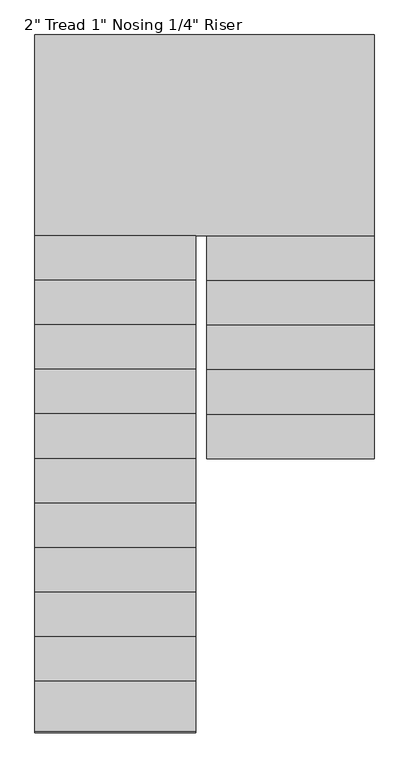
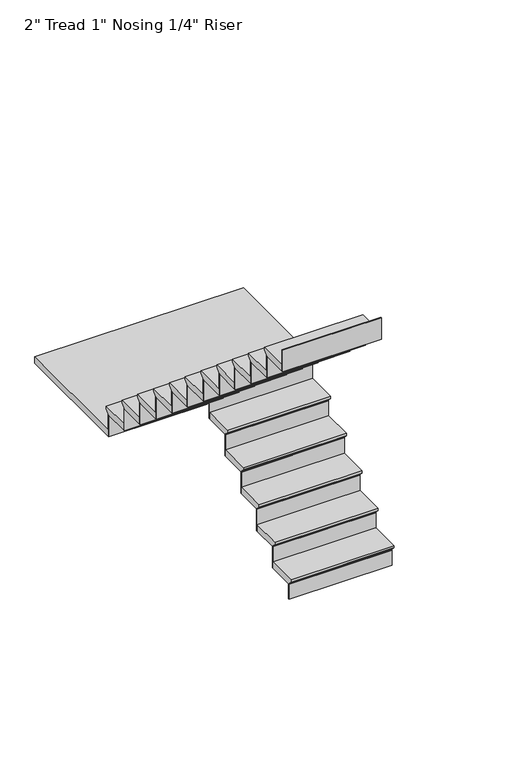
"""IFC4 building model written with IfcOpenShell, lengths in millimetres: stair flight geometry."""

from ifc_helpers import new_model, si_unit, origin, place, context, project, spatial, faceted_brep, source, transform, mapped, element, save


def stair_flight_22957a7c(model_context):
    return source(origin(), model_context, "Body", "Brep", [
        faceted_brep([(-3749.597125, 2714.6319226, 6093.8833333), (-3749.597125, 2714.6319226, 6112.9333333), (-4512.2136682, 2714.6319226, 6112.9333333), (-4512.2136682, 2714.6319226, 6093.8833333), (-3749.597125, 2740.0319226, 6068.4833333), (-4512.2136682, 2740.0319226, 6068.4833333), (-3749.597125, 2943.2319226, 6112.9333333), (-4512.2136682, 2943.2319226, 6112.9333333), (-4512.2136682, 2740.0319226, 6062.1333333), (-4512.2136682, 2943.2319226, 6062.1333333), (-3749.597125, 2943.2319226, 6062.1333333), (-3749.597125, 2740.0319226, 6062.1333333)], [[[0, 1, 2, 3]], [[4, 0, 3, 5]], [[2, 1, 6, 7]], [[8, 9, 10, 11]], [[2, 7, 9, 8, 5, 3]], [[8, 11, 4, 5]], [[6, 1, 0, 4, 11, 10]], [[7, 6, 10, 9]]]),
        faceted_brep([(-3749.597125, 2740.0319226, 6062.1333333), (-3749.597125, 2740.0319226, 5943.6), (-3749.597125, 2746.3819226, 5943.6), (-3749.597125, 2746.3819226, 6062.1333333), (-4512.2136682, 2740.0319226, 6062.1333333), (-4512.2136682, 2746.3819226, 6062.1333333), (-4512.2136682, 2746.3819226, 5943.6), (-4512.2136682, 2740.0319226, 5943.6)], [[[0, 1, 2, 3]], [[4, 5, 6, 7]], [[1, 0, 4, 7]], [[2, 1, 7, 6]], [[3, 2, 6, 5]], [[0, 3, 5, 4]]]),
        faceted_brep([(-3749.597125, 2943.2319226, 6231.4666667), (-3749.597125, 2943.2319226, 6062.1333333), (-3749.597125, 2949.5819226, 6062.1333333), (-3749.597125, 2949.5819226, 6231.4666667), (-4512.2136682, 2943.2319226, 6231.4666667), (-4512.2136682, 2949.5819226, 6231.4666667), (-4512.2136682, 2949.5819226, 6062.1333333), (-4512.2136682, 2943.2319226, 6062.1333333)], [[[0, 1, 2, 3]], [[4, 5, 6, 7]], [[1, 0, 4, 7]], [[2, 1, 7, 6]], [[3, 2, 6, 5]], [[0, 3, 5, 4]]]),
        faceted_brep([(-4512.2136682, 2917.8319226, 6282.2666667), (-3749.597125, 2917.8319226, 6282.2666667), (-3749.597125, 3146.4319226, 6282.2666667), (-4512.2136682, 3146.4319226, 6282.2666667), (-4512.2136682, 2943.2319226, 6231.4666667), (-4512.2136682, 3146.4319226, 6231.4666667), (-3749.597125, 3146.4319226, 6231.4666667), (-3749.597125, 2943.2319226, 6231.4666667), (-4512.2136682, 2943.2319226, 6237.8166667), (-4512.2136682, 2917.8319226, 6263.2166667), (-3749.597125, 2943.2319226, 6237.8166667), (-3749.597125, 2917.8319226, 6263.2166667)], [[[0, 1, 2, 3]], [[4, 5, 6, 7]], [[0, 3, 5, 4, 8, 9]], [[4, 7, 10, 8]], [[2, 1, 11, 10, 7, 6]], [[3, 2, 6, 5]], [[11, 1, 0, 9]], [[10, 11, 9, 8]]]),
        faceted_brep([(-3749.597125, 3146.4319226, 6400.8), (-3749.597125, 3146.4319226, 6231.4666667), (-3749.597125, 3152.7819226, 6231.4666667), (-3749.597125, 3152.7819226, 6400.8), (-4512.2136682, 3146.4319226, 6400.8), (-4512.2136682, 3152.7819226, 6400.8), (-4512.2136682, 3152.7819226, 6231.4666667), (-4512.2136682, 3146.4319226, 6231.4666667)], [[[0, 1, 2, 3]], [[4, 5, 6, 7]], [[1, 0, 4, 7]], [[2, 1, 7, 6]], [[3, 2, 6, 5]], [[0, 3, 5, 4]]]),
        faceted_brep([(-4512.2136682, 3121.0319226, 6451.6), (-3749.597125, 3121.0319226, 6451.6), (-3749.597125, 3349.6319226, 6451.6), (-4512.2136682, 3349.6319226, 6451.6), (-4512.2136682, 3146.4319226, 6400.8), (-4512.2136682, 3349.6319226, 6400.8), (-3749.597125, 3349.6319226, 6400.8), (-3749.597125, 3146.4319226, 6400.8), (-4512.2136682, 3146.4319226, 6407.15), (-4512.2136682, 3121.0319226, 6432.55), (-3749.597125, 3146.4319226, 6407.15), (-3749.597125, 3121.0319226, 6432.55)], [[[0, 1, 2, 3]], [[4, 5, 6, 7]], [[0, 3, 5, 4, 8, 9]], [[4, 7, 10, 8]], [[2, 1, 11, 10, 7, 6]], [[3, 2, 6, 5]], [[11, 1, 0, 9]], [[10, 11, 9, 8]]]),
        faceted_brep([(-3749.597125, 3349.6319226, 6570.1333333), (-3749.597125, 3349.6319226, 6400.8), (-3749.597125, 3355.9819226, 6400.8), (-3749.597125, 3355.9819226, 6570.1333333), (-4512.2136682, 3349.6319226, 6570.1333333), (-4512.2136682, 3355.9819226, 6570.1333333), (-4512.2136682, 3355.9819226, 6400.8), (-4512.2136682, 3349.6319226, 6400.8)], [[[0, 1, 2, 3]], [[4, 5, 6, 7]], [[1, 0, 4, 7]], [[2, 1, 7, 6]], [[3, 2, 6, 5]], [[0, 3, 5, 4]]]),
        faceted_brep([(-4512.2136682, 3324.2319226, 6620.9333333), (-3749.597125, 3324.2319226, 6620.9333333), (-3749.597125, 3552.8319226, 6620.9333333), (-4512.2136682, 3552.8319226, 6620.9333333), (-4512.2136682, 3349.6319226, 6570.1333333), (-4512.2136682, 3552.8319226, 6570.1333333), (-3749.597125, 3552.8319226, 6570.1333333), (-3749.597125, 3349.6319226, 6570.1333333), (-4512.2136682, 3349.6319226, 6576.4833333), (-4512.2136682, 3324.2319226, 6601.8833333), (-3749.597125, 3349.6319226, 6576.4833333), (-3749.597125, 3324.2319226, 6601.8833333)], [[[0, 1, 2, 3]], [[4, 5, 6, 7]], [[0, 3, 5, 4, 8, 9]], [[4, 7, 10, 8]], [[2, 1, 11, 10, 7, 6]], [[3, 2, 6, 5]], [[11, 1, 0, 9]], [[10, 11, 9, 8]]]),
        faceted_brep([(-3749.597125, 3552.8319226, 6739.4666667), (-3749.597125, 3552.8319226, 6570.1333333), (-3749.597125, 3559.1819226, 6570.1333333), (-3749.597125, 3559.1819226, 6739.4666667), (-4512.2136682, 3552.8319226, 6739.4666667), (-4512.2136682, 3559.1819226, 6739.4666667), (-4512.2136682, 3559.1819226, 6570.1333333), (-4512.2136682, 3552.8319226, 6570.1333333)], [[[0, 1, 2, 3]], [[4, 5, 6, 7]], [[1, 0, 4, 7]], [[2, 1, 7, 6]], [[3, 2, 6, 5]], [[0, 3, 5, 4]]]),
        faceted_brep([(-4512.2136682, 3527.4319226, 6790.2666667), (-3749.597125, 3527.4319226, 6790.2666667), (-3749.597125, 3756.0319226, 6790.2666667), (-4512.2136682, 3756.0319226, 6790.2666667), (-4512.2136682, 3552.8319226, 6739.4666667), (-4512.2136682, 3756.0319226, 6739.4666667), (-3749.597125, 3756.0319226, 6739.4666667), (-3749.597125, 3552.8319226, 6739.4666667), (-4512.2136682, 3552.8319226, 6745.8166667), (-4512.2136682, 3527.4319226, 6771.2166667), (-3749.597125, 3552.8319226, 6745.8166667), (-3749.597125, 3527.4319226, 6771.2166667)], [[[0, 1, 2, 3]], [[4, 5, 6, 7]], [[0, 3, 5, 4, 8, 9]], [[4, 7, 10, 8]], [[2, 1, 11, 10, 7, 6]], [[3, 2, 6, 5]], [[11, 1, 0, 9]], [[10, 11, 9, 8]]]),
        faceted_brep([(-3749.597125, 3756.0319226, 6908.8), (-3749.597125, 3756.0319226, 6739.4666667), (-3749.597125, 3762.3819226, 6739.4666667), (-3749.597125, 3762.3819226, 6908.8), (-4512.2136682, 3756.0319226, 6908.8), (-4512.2136682, 3762.3819226, 6908.8), (-4512.2136682, 3762.3819226, 6739.4666667), (-4512.2136682, 3756.0319226, 6739.4666667)], [[[0, 1, 2, 3]], [[4, 5, 6, 7]], [[1, 0, 4, 7]], [[2, 1, 7, 6]], [[3, 2, 6, 5]], [[0, 3, 5, 4]]]),
        faceted_brep([(-4563.0136682, 3705.2319226, 6959.6), (-4563.0136682, 3730.6319226, 6959.6), (-3749.597125, 3730.6319226, 6959.6), (-3749.597125, 4645.0319226, 6959.6), (-5295.0246464, 4645.0319226, 6959.6), (-5295.0246464, 3705.2319226, 6959.6), (-4563.0136682, 3730.6319226, 6908.8), (-4563.0136682, 3705.2319226, 6908.8), (-5295.0246464, 3705.2319226, 6908.8), (-5295.0246464, 4645.0319226, 6908.8), (-3749.597125, 4645.0319226, 6908.8), (-3749.597125, 3756.0319226, 6908.8), (-4512.2136682, 3756.0319226, 6908.8), (-4512.2136682, 3730.6319226, 6908.8), (-4512.2136682, 3730.6319226, 6940.55), (-3749.597125, 3730.6319226, 6940.55), (-4512.2136682, 3756.0319226, 6915.15), (-3749.597125, 3756.0319226, 6915.15)], [[[0, 1, 2, 3, 4, 5]], [[6, 7, 8, 9, 10, 11, 12, 13]], [[1, 0, 7, 6]], [[2, 1, 6, 13, 14, 15]], [[13, 12, 16, 14]], [[12, 11, 17, 16]], [[3, 2, 15, 17, 11, 10]], [[4, 3, 10, 9]], [[5, 4, 9, 8]], [[0, 5, 8, 7]], [[17, 15, 14, 16]]]),
        faceted_brep([(-5295.0246464, 3705.2319226, 7078.1333333), (-5295.0246464, 3705.2319226, 6908.8), (-5295.0246464, 3698.8819226, 6908.8), (-5295.0246464, 3698.8819226, 7078.1333333), (-4563.0136682, 3705.2319226, 7078.1333333), (-4563.0136682, 3698.8819226, 7078.1333333), (-4563.0136682, 3698.8819226, 6908.8), (-4563.0136682, 3705.2319226, 6908.8)], [[[0, 1, 2, 3]], [[4, 5, 6, 7]], [[1, 0, 4, 7]], [[2, 1, 7, 6]], [[3, 2, 6, 5]], [[0, 3, 5, 4]]]),
        faceted_brep([(-4563.0136682, 3730.6319226, 7128.9333333), (-5295.0246464, 3730.6319226, 7128.9333333), (-5295.0246464, 3502.0319226, 7128.9333333), (-4563.0136682, 3502.0319226, 7128.9333333), (-4563.0136682, 3705.2319226, 7078.1333333), (-4563.0136682, 3502.0319226, 7078.1333333), (-5295.0246464, 3502.0319226, 7078.1333333), (-5295.0246464, 3705.2319226, 7078.1333333), (-4563.0136682, 3705.2319226, 7084.4833333), (-4563.0136682, 3730.6319226, 7109.8833333), (-5295.0246464, 3705.2319226, 7084.4833333), (-5295.0246464, 3730.6319226, 7109.8833333)], [[[0, 1, 2, 3]], [[4, 5, 6, 7]], [[0, 3, 5, 4, 8, 9]], [[4, 7, 10, 8]], [[2, 1, 11, 10, 7, 6]], [[3, 2, 6, 5]], [[11, 1, 0, 9]], [[10, 11, 9, 8]]]),
        faceted_brep([(-5295.0246464, 3502.0319226, 7247.4666667), (-5295.0246464, 3502.0319226, 7078.1333333), (-5295.0246464, 3495.6819226, 7078.1333333), (-5295.0246464, 3495.6819226, 7247.4666667), (-4563.0136682, 3502.0319226, 7247.4666667), (-4563.0136682, 3495.6819226, 7247.4666667), (-4563.0136682, 3495.6819226, 7078.1333333), (-4563.0136682, 3502.0319226, 7078.1333333)], [[[0, 1, 2, 3]], [[4, 5, 6, 7]], [[1, 0, 4, 7]], [[2, 1, 7, 6]], [[3, 2, 6, 5]], [[0, 3, 5, 4]]]),
        faceted_brep([(-4563.0136682, 3527.4319226, 7298.2666667), (-5295.0246464, 3527.4319226, 7298.2666667), (-5295.0246464, 3298.8319226, 7298.2666667), (-4563.0136682, 3298.8319226, 7298.2666667), (-4563.0136682, 3502.0319226, 7247.4666667), (-4563.0136682, 3298.8319226, 7247.4666667), (-5295.0246464, 3298.8319226, 7247.4666667), (-5295.0246464, 3502.0319226, 7247.4666667), (-4563.0136682, 3502.0319226, 7253.8166667), (-4563.0136682, 3527.4319226, 7279.2166667), (-5295.0246464, 3502.0319226, 7253.8166667), (-5295.0246464, 3527.4319226, 7279.2166667)], [[[0, 1, 2, 3]], [[4, 5, 6, 7]], [[0, 3, 5, 4, 8, 9]], [[4, 7, 10, 8]], [[2, 1, 11, 10, 7, 6]], [[3, 2, 6, 5]], [[11, 1, 0, 9]], [[10, 11, 9, 8]]]),
        faceted_brep([(-5295.0246464, 3298.8319226, 7416.8), (-5295.0246464, 3298.8319226, 7247.4666667), (-5295.0246464, 3292.4819226, 7247.4666667), (-5295.0246464, 3292.4819226, 7416.8), (-4563.0136682, 3298.8319226, 7416.8), (-4563.0136682, 3292.4819226, 7416.8), (-4563.0136682, 3292.4819226, 7247.4666667), (-4563.0136682, 3298.8319226, 7247.4666667)], [[[0, 1, 2, 3]], [[4, 5, 6, 7]], [[1, 0, 4, 7]], [[2, 1, 7, 6]], [[3, 2, 6, 5]], [[0, 3, 5, 4]]]),
        faceted_brep([(-4563.0136682, 3324.2319226, 7467.6), (-5295.0246464, 3324.2319226, 7467.6), (-5295.0246464, 3095.6319226, 7467.6), (-4563.0136682, 3095.6319226, 7467.6), (-4563.0136682, 3298.8319226, 7416.8), (-4563.0136682, 3095.6319226, 7416.8), (-5295.0246464, 3095.6319226, 7416.8), (-5295.0246464, 3298.8319226, 7416.8), (-4563.0136682, 3298.8319226, 7423.15), (-4563.0136682, 3324.2319226, 7448.55), (-5295.0246464, 3298.8319226, 7423.15), (-5295.0246464, 3324.2319226, 7448.55)], [[[0, 1, 2, 3]], [[4, 5, 6, 7]], [[0, 3, 5, 4, 8, 9]], [[4, 7, 10, 8]], [[2, 1, 11, 10, 7, 6]], [[3, 2, 6, 5]], [[11, 1, 0, 9]], [[10, 11, 9, 8]]]),
        faceted_brep([(-5295.0246464, 3095.6319226, 7586.1333333), (-5295.0246464, 3095.6319226, 7416.8), (-5295.0246464, 3089.2819226, 7416.8), (-5295.0246464, 3089.2819226, 7586.1333333), (-4563.0136682, 3095.6319226, 7586.1333333), (-4563.0136682, 3089.2819226, 7586.1333333), (-4563.0136682, 3089.2819226, 7416.8), (-4563.0136682, 3095.6319226, 7416.8)], [[[0, 1, 2, 3]], [[4, 5, 6, 7]], [[1, 0, 4, 7]], [[2, 1, 7, 6]], [[3, 2, 6, 5]], [[0, 3, 5, 4]]]),
        faceted_brep([(-4563.0136682, 3121.0319226, 7636.9333333), (-5295.0246464, 3121.0319226, 7636.9333333), (-5295.0246464, 2892.4319226, 7636.9333333), (-4563.0136682, 2892.4319226, 7636.9333333), (-4563.0136682, 3095.6319226, 7586.1333333), (-4563.0136682, 2892.4319226, 7586.1333333), (-5295.0246464, 2892.4319226, 7586.1333333), (-5295.0246464, 3095.6319226, 7586.1333333), (-4563.0136682, 3095.6319226, 7592.4833333), (-4563.0136682, 3121.0319226, 7617.8833333), (-5295.0246464, 3095.6319226, 7592.4833333), (-5295.0246464, 3121.0319226, 7617.8833333)], [[[0, 1, 2, 3]], [[4, 5, 6, 7]], [[0, 3, 5, 4, 8, 9]], [[4, 7, 10, 8]], [[2, 1, 11, 10, 7, 6]], [[3, 2, 6, 5]], [[11, 1, 0, 9]], [[10, 11, 9, 8]]]),
        faceted_brep([(-5295.0246464, 2892.4319226, 7755.4666667), (-5295.0246464, 2892.4319226, 7586.1333333), (-5295.0246464, 2886.0819226, 7586.1333333), (-5295.0246464, 2886.0819226, 7755.4666667), (-4563.0136682, 2892.4319226, 7755.4666667), (-4563.0136682, 2886.0819226, 7755.4666667), (-4563.0136682, 2886.0819226, 7586.1333333), (-4563.0136682, 2892.4319226, 7586.1333333)], [[[0, 1, 2, 3]], [[4, 5, 6, 7]], [[1, 0, 4, 7]], [[2, 1, 7, 6]], [[3, 2, 6, 5]], [[0, 3, 5, 4]]]),
        faceted_brep([(-4563.0136682, 2917.8319226, 7806.2666667), (-5295.0246464, 2917.8319226, 7806.2666667), (-5295.0246464, 2689.2319226, 7806.2666667), (-4563.0136682, 2689.2319226, 7806.2666667), (-4563.0136682, 2892.4319226, 7755.4666667), (-4563.0136682, 2689.2319226, 7755.4666667), (-5295.0246464, 2689.2319226, 7755.4666667), (-5295.0246464, 2892.4319226, 7755.4666667), (-4563.0136682, 2892.4319226, 7761.8166667), (-4563.0136682, 2917.8319226, 7787.2166667), (-5295.0246464, 2892.4319226, 7761.8166667), (-5295.0246464, 2917.8319226, 7787.2166667)], [[[0, 1, 2, 3]], [[4, 5, 6, 7]], [[0, 3, 5, 4, 8, 9]], [[4, 7, 10, 8]], [[2, 1, 11, 10, 7, 6]], [[3, 2, 6, 5]], [[11, 1, 0, 9]], [[10, 11, 9, 8]]]),
        faceted_brep([(-5295.0246464, 2689.2319226, 7924.8), (-5295.0246464, 2689.2319226, 7755.4666667), (-5295.0246464, 2682.8819226, 7755.4666667), (-5295.0246464, 2682.8819226, 7924.8), (-4563.0136682, 2689.2319226, 7924.8), (-4563.0136682, 2682.8819226, 7924.8), (-4563.0136682, 2682.8819226, 7755.4666667), (-4563.0136682, 2689.2319226, 7755.4666667)], [[[0, 1, 2, 3]], [[4, 5, 6, 7]], [[1, 0, 4, 7]], [[2, 1, 7, 6]], [[3, 2, 6, 5]], [[0, 3, 5, 4]]]),
        faceted_brep([(-4563.0136682, 2714.6319226, 7975.6), (-5295.0246464, 2714.6319226, 7975.6), (-5295.0246464, 2486.0319226, 7975.6), (-4563.0136682, 2486.0319226, 7975.6), (-4563.0136682, 2689.2319226, 7924.8), (-4563.0136682, 2486.0319226, 7924.8), (-5295.0246464, 2486.0319226, 7924.8), (-5295.0246464, 2689.2319226, 7924.8), (-4563.0136682, 2689.2319226, 7931.15), (-4563.0136682, 2714.6319226, 7956.55), (-5295.0246464, 2689.2319226, 7931.15), (-5295.0246464, 2714.6319226, 7956.55)], [[[0, 1, 2, 3]], [[4, 5, 6, 7]], [[0, 3, 5, 4, 8, 9]], [[4, 7, 10, 8]], [[2, 1, 11, 10, 7, 6]], [[3, 2, 6, 5]], [[11, 1, 0, 9]], [[10, 11, 9, 8]]]),
        faceted_brep([(-5295.0246464, 2486.0319226, 8094.1333333), (-5295.0246464, 2486.0319226, 7924.8), (-5295.0246464, 2479.6819226, 7924.8), (-5295.0246464, 2479.6819226, 8094.1333333), (-4563.0136682, 2486.0319226, 8094.1333333), (-4563.0136682, 2479.6819226, 8094.1333333), (-4563.0136682, 2479.6819226, 7924.8), (-4563.0136682, 2486.0319226, 7924.8)], [[[0, 1, 2, 3]], [[4, 5, 6, 7]], [[1, 0, 4, 7]], [[2, 1, 7, 6]], [[3, 2, 6, 5]], [[0, 3, 5, 4]]]),
        faceted_brep([(-4563.0136682, 2511.4319226, 8144.9333333), (-5295.0246464, 2511.4319226, 8144.9333333), (-5295.0246464, 2282.8319226, 8144.9333333), (-4563.0136682, 2282.8319226, 8144.9333333), (-4563.0136682, 2486.0319226, 8094.1333333), (-4563.0136682, 2282.8319226, 8094.1333333), (-5295.0246464, 2282.8319226, 8094.1333333), (-5295.0246464, 2486.0319226, 8094.1333333), (-4563.0136682, 2486.0319226, 8100.4833333), (-4563.0136682, 2511.4319226, 8125.8833333), (-5295.0246464, 2486.0319226, 8100.4833333), (-5295.0246464, 2511.4319226, 8125.8833333)], [[[0, 1, 2, 3]], [[4, 5, 6, 7]], [[0, 3, 5, 4, 8, 9]], [[4, 7, 10, 8]], [[2, 1, 11, 10, 7, 6]], [[3, 2, 6, 5]], [[11, 1, 0, 9]], [[10, 11, 9, 8]]]),
        faceted_brep([(-5295.0246464, 2282.8319226, 8263.4666667), (-5295.0246464, 2282.8319226, 8094.1333333), (-5295.0246464, 2276.4819226, 8094.1333333), (-5295.0246464, 2276.4819226, 8263.4666667), (-4563.0136682, 2282.8319226, 8263.4666667), (-4563.0136682, 2276.4819226, 8263.4666667), (-4563.0136682, 2276.4819226, 8094.1333333), (-4563.0136682, 2282.8319226, 8094.1333333)], [[[0, 1, 2, 3]], [[4, 5, 6, 7]], [[1, 0, 4, 7]], [[2, 1, 7, 6]], [[3, 2, 6, 5]], [[0, 3, 5, 4]]]),
        faceted_brep([(-4563.0136682, 2308.2319226, 8314.2666667), (-5295.0246464, 2308.2319226, 8314.2666667), (-5295.0246464, 2079.6319226, 8314.2666667), (-4563.0136682, 2079.6319226, 8314.2666667), (-4563.0136682, 2282.8319226, 8263.4666667), (-4563.0136682, 2079.6319226, 8263.4666667), (-5295.0246464, 2079.6319226, 8263.4666667), (-5295.0246464, 2282.8319226, 8263.4666667), (-4563.0136682, 2282.8319226, 8269.8166667), (-4563.0136682, 2308.2319226, 8295.2166667), (-5295.0246464, 2282.8319226, 8269.8166667), (-5295.0246464, 2308.2319226, 8295.2166667)], [[[0, 1, 2, 3]], [[4, 5, 6, 7]], [[0, 3, 5, 4, 8, 9]], [[4, 7, 10, 8]], [[2, 1, 11, 10, 7, 6]], [[3, 2, 6, 5]], [[11, 1, 0, 9]], [[10, 11, 9, 8]]]),
        faceted_brep([(-5295.0246464, 2079.6319226, 8432.8), (-5295.0246464, 2079.6319226, 8263.4666667), (-5295.0246464, 2073.2819226, 8263.4666667), (-5295.0246464, 2073.2819226, 8432.8), (-4563.0136682, 2079.6319226, 8432.8), (-4563.0136682, 2073.2819226, 8432.8), (-4563.0136682, 2073.2819226, 8263.4666667), (-4563.0136682, 2079.6319226, 8263.4666667)], [[[0, 1, 2, 3]], [[4, 5, 6, 7]], [[1, 0, 4, 7]], [[2, 1, 7, 6]], [[3, 2, 6, 5]], [[0, 3, 5, 4]]]),
        faceted_brep([(-4563.0136682, 2105.0319226, 8483.6), (-5295.0246464, 2105.0319226, 8483.6), (-5295.0246464, 1876.4319226, 8483.6), (-4563.0136682, 1876.4319226, 8483.6), (-4563.0136682, 2079.6319226, 8432.8), (-4563.0136682, 1876.4319226, 8432.8), (-5295.0246464, 1876.4319226, 8432.8), (-5295.0246464, 2079.6319226, 8432.8), (-4563.0136682, 2079.6319226, 8439.15), (-4563.0136682, 2105.0319226, 8464.55), (-5295.0246464, 2079.6319226, 8439.15), (-5295.0246464, 2105.0319226, 8464.55)], [[[0, 1, 2, 3]], [[4, 5, 6, 7]], [[0, 3, 5, 4, 8, 9]], [[4, 7, 10, 8]], [[2, 1, 11, 10, 7, 6]], [[3, 2, 6, 5]], [[11, 1, 0, 9]], [[10, 11, 9, 8]]]),
        faceted_brep([(-5295.0246464, 1876.4319226, 8602.1333333), (-5295.0246464, 1876.4319226, 8432.8), (-5295.0246464, 1870.0819226, 8432.8), (-5295.0246464, 1870.0819226, 8602.1333333), (-4563.0136682, 1876.4319226, 8602.1333333), (-4563.0136682, 1870.0819226, 8602.1333333), (-4563.0136682, 1870.0819226, 8432.8), (-4563.0136682, 1876.4319226, 8432.8)], [[[0, 1, 2, 3]], [[4, 5, 6, 7]], [[1, 0, 4, 7]], [[2, 1, 7, 6]], [[3, 2, 6, 5]], [[0, 3, 5, 4]]]),
        faceted_brep([(-4563.0136682, 1901.8319226, 8652.9333333), (-5295.0246464, 1901.8319226, 8652.9333333), (-5295.0246464, 1673.2319226, 8652.9333333), (-4563.0136682, 1673.2319226, 8652.9333333), (-4563.0136682, 1876.4319226, 8602.1333333), (-4563.0136682, 1673.2319226, 8602.1333333), (-5295.0246464, 1673.2319226, 8602.1333333), (-5295.0246464, 1876.4319226, 8602.1333333), (-4563.0136682, 1876.4319226, 8608.4833333), (-4563.0136682, 1901.8319226, 8633.8833333), (-5295.0246464, 1876.4319226, 8608.4833333), (-5295.0246464, 1901.8319226, 8633.8833333)], [[[0, 1, 2, 3]], [[4, 5, 6, 7]], [[0, 3, 5, 4, 8, 9]], [[4, 7, 10, 8]], [[2, 1, 11, 10, 7, 6]], [[3, 2, 6, 5]], [[11, 1, 0, 9]], [[10, 11, 9, 8]]]),
        faceted_brep([(-5295.0246464, 1673.2319226, 8771.4666667), (-5295.0246464, 1673.2319226, 8602.1333333), (-5295.0246464, 1666.8819226, 8602.1333333), (-5295.0246464, 1666.8819226, 8771.4666667), (-4563.0136682, 1673.2319226, 8771.4666667), (-4563.0136682, 1666.8819226, 8771.4666667), (-4563.0136682, 1666.8819226, 8602.1333333), (-4563.0136682, 1673.2319226, 8602.1333333)], [[[0, 1, 2, 3]], [[4, 5, 6, 7]], [[1, 0, 4, 7]], [[2, 1, 7, 6]], [[3, 2, 6, 5]], [[0, 3, 5, 4]]]),
        faceted_brep([(-4563.0136682, 1698.6319226, 8822.2666667), (-5295.0246464, 1698.6319226, 8822.2666667), (-5295.0246464, 1470.0319226, 8822.2666667), (-4563.0136682, 1470.0319226, 8822.2666667), (-4563.0136682, 1673.2319226, 8771.4666667), (-4563.0136682, 1470.0319226, 8771.4666667), (-5295.0246464, 1470.0319226, 8771.4666667), (-5295.0246464, 1673.2319226, 8771.4666667), (-4563.0136682, 1673.2319226, 8777.8166667), (-4563.0136682, 1698.6319226, 8803.2166667), (-5295.0246464, 1673.2319226, 8777.8166667), (-5295.0246464, 1698.6319226, 8803.2166667)], [[[0, 1, 2, 3]], [[4, 5, 6, 7]], [[0, 3, 5, 4, 8, 9]], [[4, 7, 10, 8]], [[2, 1, 11, 10, 7, 6]], [[3, 2, 6, 5]], [[11, 1, 0, 9]], [[10, 11, 9, 8]]]),
        faceted_brep([(-5295.0246464, 1470.0319226, 8940.8), (-5295.0246464, 1470.0319226, 8771.4666667), (-5295.0246464, 1463.6819226, 8771.4666667), (-5295.0246464, 1463.6819226, 8940.8), (-4563.0136682, 1470.0319226, 8940.8), (-4563.0136682, 1463.6819226, 8940.8), (-4563.0136682, 1463.6819226, 8771.4666667), (-4563.0136682, 1470.0319226, 8771.4666667)], [[[0, 1, 2, 3]], [[4, 5, 6, 7]], [[1, 0, 4, 7]], [[2, 1, 7, 6]], [[3, 2, 6, 5]], [[0, 3, 5, 4]]]),
    ])


if __name__ == "__main__":
    model = new_model("IFC4")
    model_context = context("Model", 3, world=origin())
    ifc_project = project(units=[si_unit("LENGTHUNIT", "METRE", prefix="MILLI")], contexts=[model_context])
    site = spatial("IfcSite", under=ifc_project)
    building = spatial("IfcBuilding", under=site)
    placement = place(None, origin())
    stair_flight_shape = stair_flight_22957a7c(model_context)
    element("IfcStairFlight", 1, ObjectType="2\" Tread 1\" Nosing 1/4\" Riser", at=placement, inside=building, context=model_context, shape_type="MappedRepresentation", body=[
        mapped(stair_flight_shape, transform((0.0, 0.0, 0.0), x_axis=(1.0, 0.0, 0.0), y_axis=(0.0, 1.0, 0.0), z_axis=(0.0, 0.0, 1.0))),
    ])
    save(model, "model.ifc")
